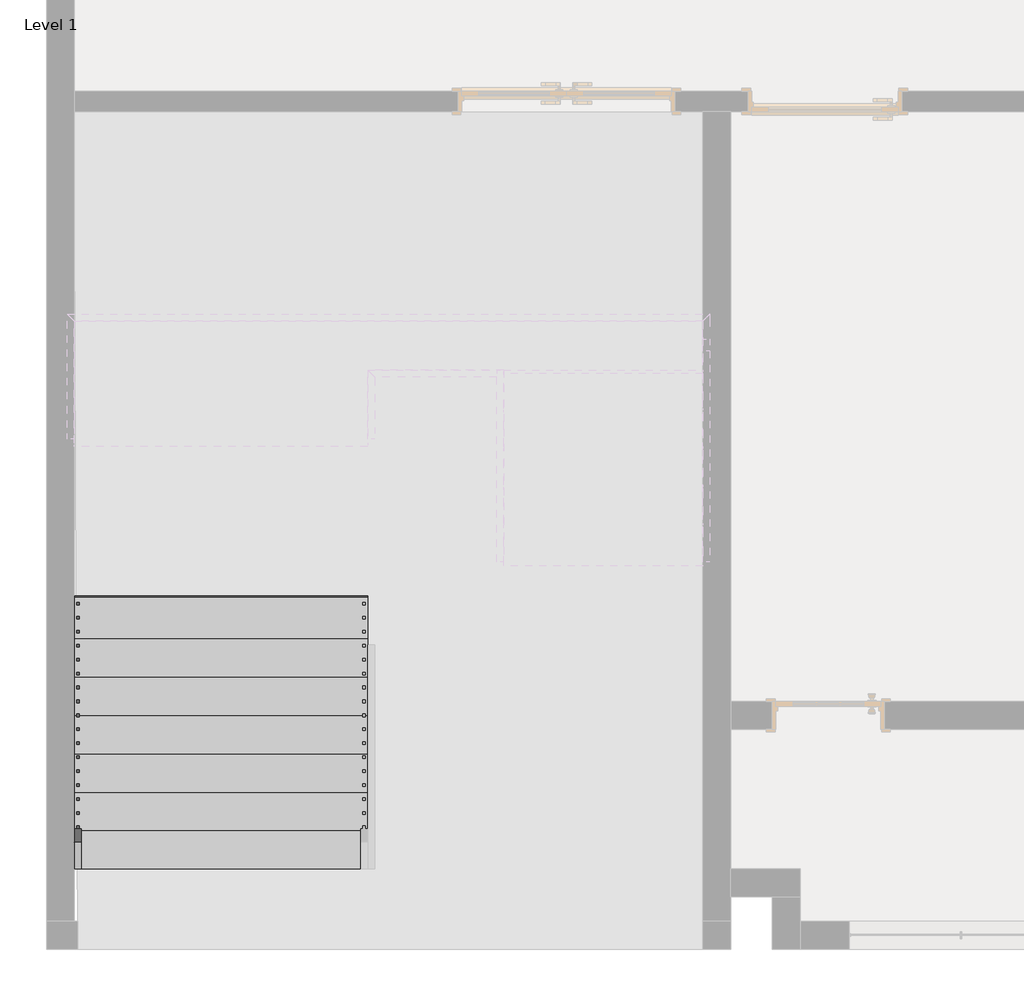
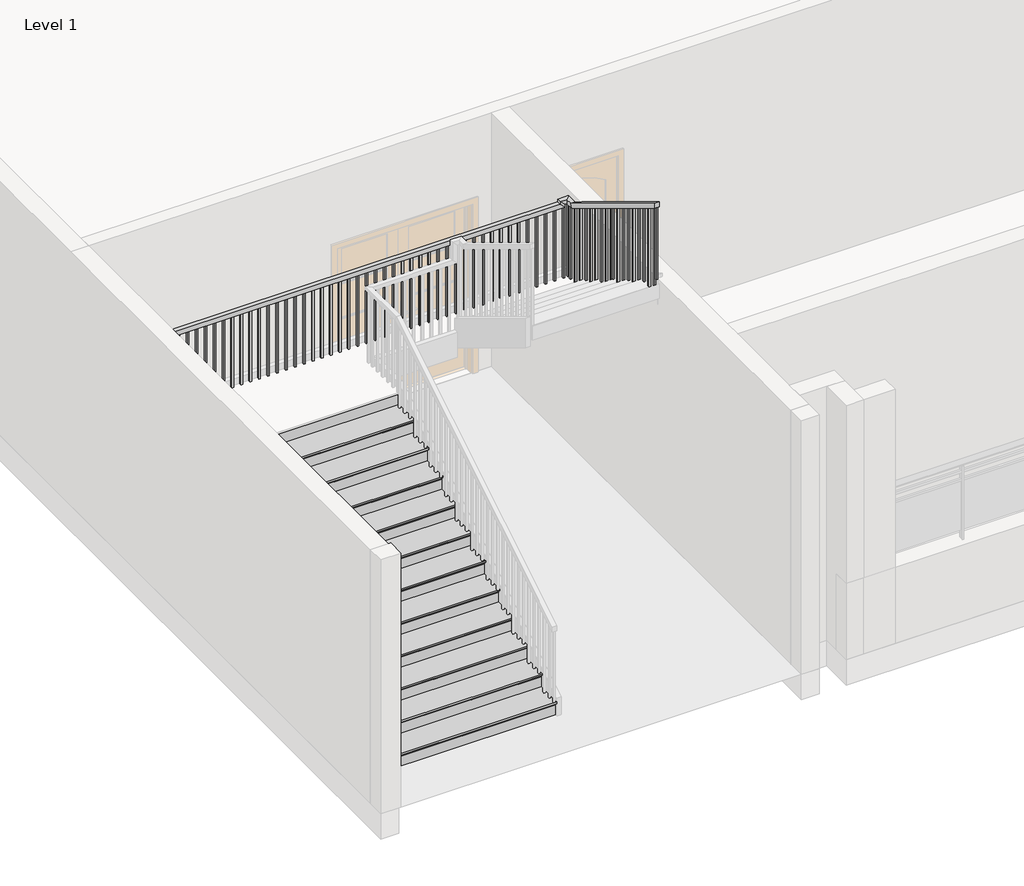
# One storey, part 3 of 4: 1 railing, 1 stair flight.
"""IFC4 building model written with IfcOpenShell, lengths in millimetres."""

from ifc_helpers import new_model, si_unit, frame, origin, place, context, project, spatial, polyline, outline, extrude, faceted_brep, transform, mapped, element, save
from components import stair_flight_3e597512

model = new_model("IFC4")

# Units and contexts
model_context = context("Model", 3, world=origin())
ifc_project = project(units=[si_unit("LENGTHUNIT", "METRE", prefix="MILLI")], contexts=[model_context])

# Site, building, storey
site = spatial("IfcSite", under=ifc_project)
building = spatial("IfcBuilding", under=site)
storey = spatial("IfcBuildingStorey", under=building, Name="Level 1", Elevation=0.0)

# Railing
placement = place(None, origin())
element("IfcRailing", 1, ObjectType="Handrail - Rectangular", at=placement, inside=storey, context=model_context, shape_type="SolidModel", body=[
    faceted_brep([(-19977.2480019, -193.7741123, 1083.7333333), (-19977.2480019, -193.7741123, 1024.3318731), (-19926.4480019, -193.7741123, 1024.3318731), (-19926.4480019, -193.7741123, 1083.7333333), (-19977.2480019, 2879.6258877, 2946.4), (-19977.2480019, 2893.8182972, 2895.6), (-19926.4480019, 2893.8182972, 2895.6), (-19926.4480019, 2879.6258877, 2946.4), (-19977.2480019, 3794.0258877, 2946.4), (-19977.2480019, 3794.0258877, 2895.6), (-19926.4480019, 3743.2258877, 2895.6), (-19926.4480019, 3743.2258877, 2946.4), (-15532.2480019, 3794.0258877, 2946.4), (-15481.4480019, 3794.0258877, 2895.6), (-15481.4480019, 3743.2258877, 2895.6), (-15532.2480019, 3743.2258877, 2946.4), (-15405.2480019, 2016.0258877, 3977.7939394), (-15456.0480019, 2016.0258877, 3977.7939394), (-15456.0480019, 2016.0258877, 3918.3924791), (-15405.2480019, 2016.0258877, 3918.3924791), (-15405.2480019, 3652.8334783, 2926.3878788), (-15405.2480019, 3667.0258877, 2977.1878788), (-15456.0480019, 3652.8334783, 2926.3878788), (-15456.0480019, 3667.0258877, 2977.1878788), (-15532.2480019, 3794.0258877, 2977.1878788), (-15481.4480019, 3794.0258877, 2926.3878788), (-15481.4480019, 3743.2258877, 2926.3878788), (-15532.2480019, 3743.2258877, 2977.1878788), (-15405.2480019, 3794.0258877, 2977.1878788), (-15405.2480019, 3794.0258877, 2926.3878788), (-15456.0480019, 3743.2258877, 2926.3878788), (-15456.0480019, 3743.2258877, 2977.1878788)], [[[0, 1, 2, 3]], [[1, 0, 4, 5]], [[2, 1, 5, 6]], [[3, 2, 6, 7]], [[0, 3, 7, 4]], [[5, 4, 8, 9]], [[6, 5, 9, 10]], [[7, 6, 10, 11]], [[4, 7, 11, 8]], [[9, 8, 12, 13]], [[10, 9, 13, 14]], [[11, 10, 14, 15]], [[8, 11, 15, 12]], [[16, 17, 18, 19]], [[20, 21, 16, 19]], [[22, 20, 19, 18]], [[23, 22, 18, 17]], [[21, 23, 17, 16]], [[13, 12, 24, 25]], [[14, 13, 25, 26]], [[15, 14, 26, 27]], [[12, 15, 27, 24]], [[25, 24, 28, 29]], [[26, 25, 29, 30]], [[27, 26, 30, 31]], [[24, 27, 31, 28]], [[29, 28, 21, 20]], [[30, 29, 20, 22]], [[31, 30, 22, 23]], [[28, 31, 23, 21]]]),
    extrude(outline(polyline([(2076.3508877, 3881.8318731), (2076.3508877, 2878.6666667), (2057.3008877, 2878.6666667), (2057.3008877, 3893.3773276), (2076.3508877, 3881.8318731)])), frame((-15440.1730019, 0.0, 0.0), z_axis=(1.0, 0.0, 0.0), x_axis=(0.0, 1.0, 0.0)), (0.0, 0.0, 1.0), 19.05),
    extrude(outline(polyline([(2177.9508877, 3820.2561155), (2177.9508877, 2878.6666667), (2158.9008877, 2878.6666667), (2158.9008877, 3831.80157), (2177.9508877, 3820.2561155)])), frame((-15440.1730019, 0.0, 0.0), z_axis=(1.0, 0.0, 0.0), x_axis=(0.0, 1.0, 0.0)), (0.0, 0.0, 1.0), 19.05),
    extrude(outline(polyline([(2279.5508877, 3758.6803579), (2279.5508877, 2878.6666667), (2260.5008877, 2878.6666667), (2260.5008877, 3770.2258125), (2279.5508877, 3758.6803579)])), frame((-15440.1730019, 0.0, 0.0), z_axis=(1.0, 0.0, 0.0), x_axis=(0.0, 1.0, 0.0)), (0.0, 0.0, 1.0), 19.05),
    extrude(outline(polyline([(2381.1508877, 3697.1046004), (2381.1508877, 2709.3333333), (2362.1008877, 2709.3333333), (2362.1008877, 3708.6500549), (2381.1508877, 3697.1046004)])), frame((-15440.1730019, 0.0, 0.0), z_axis=(1.0, 0.0, 0.0), x_axis=(0.0, 1.0, 0.0)), (0.0, 0.0, 1.0), 19.05),
    extrude(outline(polyline([(2482.7508877, 3635.5288428), (2482.7508877, 2709.3333333), (2463.7008877, 2709.3333333), (2463.7008877, 3647.0742973), (2482.7508877, 3635.5288428)])), frame((-15440.1730019, 0.0, 0.0), z_axis=(1.0, 0.0, 0.0), x_axis=(0.0, 1.0, 0.0)), (0.0, 0.0, 1.0), 19.05),
    extrude(outline(polyline([(2584.3508877, 3573.9530852), (2584.3508877, 2709.3333333), (2565.3008877, 2709.3333333), (2565.3008877, 3585.4985397), (2584.3508877, 3573.9530852)])), frame((-15440.1730019, 0.0, 0.0), z_axis=(1.0, 0.0, 0.0), x_axis=(0.0, 1.0, 0.0)), (0.0, 0.0, 1.0), 19.05),
    extrude(outline(polyline([(2685.9508877, 3512.3773276), (2685.9508877, 2540.0), (2666.9008877, 2540.0), (2666.9008877, 3523.9227822), (2685.9508877, 3512.3773276)])), frame((-15440.1730019, 0.0, 0.0), z_axis=(1.0, 0.0, 0.0), x_axis=(0.0, 1.0, 0.0)), (0.0, 0.0, 1.0), 19.05),
    extrude(outline(polyline([(2787.5508877, 3450.80157), (2787.5508877, 2540.0), (2768.5008877, 2540.0), (2768.5008877, 3462.3470246), (2787.5508877, 3450.80157)])), frame((-15440.1730019, 0.0, 0.0), z_axis=(1.0, 0.0, 0.0), x_axis=(0.0, 1.0, 0.0)), (0.0, 0.0, 1.0), 19.05),
    extrude(outline(polyline([(2914.5508877, 3373.8318731), (2914.5508877, 2370.6666667), (2895.5008877, 2370.6666667), (2895.5008877, 3385.3773276), (2914.5508877, 3373.8318731)])), frame((-15440.1730019, 0.0, 0.0), z_axis=(1.0, 0.0, 0.0), x_axis=(0.0, 1.0, 0.0)), (0.0, 0.0, 1.0), 19.05),
    extrude(outline(polyline([(3016.1508877, 3312.2561155), (3016.1508877, 2370.6666667), (2997.1008877, 2370.6666667), (2997.1008877, 3323.80157), (3016.1508877, 3312.2561155)])), frame((-15440.1730019, 0.0, 0.0), z_axis=(1.0, 0.0, 0.0), x_axis=(0.0, 1.0, 0.0)), (0.0, 0.0, 1.0), 19.05),
    extrude(outline(polyline([(3117.7508877, 3250.6803579), (3117.7508877, 2370.6666667), (3098.7008877, 2370.6666667), (3098.7008877, 3262.2258125), (3117.7508877, 3250.6803579)])), frame((-15440.1730019, 0.0, 0.0), z_axis=(1.0, 0.0, 0.0), x_axis=(0.0, 1.0, 0.0)), (0.0, 0.0, 1.0), 19.05),
    extrude(outline(polyline([(3219.3508877, 3189.1046004), (3219.3508877, 2201.3333333), (3200.3008877, 2201.3333333), (3200.3008877, 3200.6500549), (3219.3508877, 3189.1046004)])), frame((-15440.1730019, 0.0, 0.0), z_axis=(1.0, 0.0, 0.0), x_axis=(0.0, 1.0, 0.0)), (0.0, 0.0, 1.0), 19.05),
    extrude(outline(polyline([(3320.9508877, 3127.5288428), (3320.9508877, 2201.3333333), (3301.9008877, 2201.3333333), (3301.9008877, 3139.0742973), (3320.9508877, 3127.5288428)])), frame((-15440.1730019, 0.0, 0.0), z_axis=(1.0, 0.0, 0.0), x_axis=(0.0, 1.0, 0.0)), (0.0, 0.0, 1.0), 19.05),
    extrude(outline(polyline([(3422.5508877, 3065.9530852), (3422.5508877, 2201.3333333), (3403.5008877, 2201.3333333), (3403.5008877, 3077.4985397), (3422.5508877, 3065.9530852)])), frame((-15440.1730019, 0.0, 0.0), z_axis=(1.0, 0.0, 0.0), x_axis=(0.0, 1.0, 0.0)), (0.0, 0.0, 1.0), 19.05),
    extrude(outline(polyline([(3524.1508877, 3004.3773276), (3524.1508877, 2032.0), (3505.1008877, 2032.0), (3505.1008877, 3015.9227822), (3524.1508877, 3004.3773276)])), frame((-15440.1730019, 0.0, 0.0), z_axis=(1.0, 0.0, 0.0), x_axis=(0.0, 1.0, 0.0)), (0.0, 0.0, 1.0), 19.05),
    extrude(outline(polyline([(3625.7508877, 2942.80157), (3625.7508877, 2032.0), (3606.7008877, 2032.0), (3606.7008877, 2954.3470246), (3625.7508877, 2942.80157)])), frame((-15440.1730019, 0.0, 0.0), z_axis=(1.0, 0.0, 0.0), x_axis=(0.0, 1.0, 0.0)), (0.0, 0.0, 1.0), 19.05),
    extrude(outline(polyline([(-15490.9730019, 3778.1508877), (-15471.9230019, 3778.1508877), (-15471.9230019, 3759.1008877), (-15490.9730019, 3759.1008877), (-15490.9730019, 3778.1508877)])), frame((0.0, 0.0, 2032.0), z_axis=(0.0, 0.0, 1.0), x_axis=(1.0, 0.0, 0.0)), (0.0, 0.0, 1.0), 863.6),
    extrude(outline(polyline([(-15592.5730019, 3778.1508877), (-15573.5230019, 3778.1508877), (-15573.5230019, 3759.1008877), (-15592.5730019, 3759.1008877), (-15592.5730019, 3778.1508877)])), frame((0.0, 0.0, 2032.0), z_axis=(0.0, 0.0, 1.0), x_axis=(1.0, 0.0, 0.0)), (0.0, 0.0, 1.0), 863.6),
    extrude(outline(polyline([(-15694.1730019, 3778.1508877), (-15675.1230019, 3778.1508877), (-15675.1230019, 3759.1008877), (-15694.1730019, 3759.1008877), (-15694.1730019, 3778.1508877)])), frame((0.0, 0.0, 2032.0), z_axis=(0.0, 0.0, 1.0), x_axis=(1.0, 0.0, 0.0)), (0.0, 0.0, 1.0), 863.6),
    extrude(outline(polyline([(-15795.7730019, 3778.1508877), (-15776.7230019, 3778.1508877), (-15776.7230019, 3759.1008877), (-15795.7730019, 3759.1008877), (-15795.7730019, 3778.1508877)])), frame((0.0, 0.0, 2032.0), z_axis=(0.0, 0.0, 1.0), x_axis=(1.0, 0.0, 0.0)), (0.0, 0.0, 1.0), 863.6),
    extrude(outline(polyline([(-15897.3730019, 3778.1508877), (-15878.3230019, 3778.1508877), (-15878.3230019, 3759.1008877), (-15897.3730019, 3759.1008877), (-15897.3730019, 3778.1508877)])), frame((0.0, 0.0, 2032.0), z_axis=(0.0, 0.0, 1.0), x_axis=(1.0, 0.0, 0.0)), (0.0, 0.0, 1.0), 863.6),
    extrude(outline(polyline([(-15998.9730019, 3778.1508877), (-15979.9230019, 3778.1508877), (-15979.9230019, 3759.1008877), (-15998.9730019, 3759.1008877), (-15998.9730019, 3778.1508877)])), frame((0.0, 0.0, 2032.0), z_axis=(0.0, 0.0, 1.0), x_axis=(1.0, 0.0, 0.0)), (0.0, 0.0, 1.0), 863.6),
    extrude(outline(polyline([(-16100.5730019, 3778.1508877), (-16081.5230019, 3778.1508877), (-16081.5230019, 3759.1008877), (-16100.5730019, 3759.1008877), (-16100.5730019, 3778.1508877)])), frame((0.0, 0.0, 2032.0), z_axis=(0.0, 0.0, 1.0), x_axis=(1.0, 0.0, 0.0)), (0.0, 0.0, 1.0), 863.6),
    extrude(outline(polyline([(-16202.1730019, 3778.1508877), (-16183.1230019, 3778.1508877), (-16183.1230019, 3759.1008877), (-16202.1730019, 3759.1008877), (-16202.1730019, 3778.1508877)])), frame((0.0, 0.0, 2032.0), z_axis=(0.0, 0.0, 1.0), x_axis=(1.0, 0.0, 0.0)), (0.0, 0.0, 1.0), 863.6),
    extrude(outline(polyline([(-16303.7730019, 3778.1508877), (-16284.7230019, 3778.1508877), (-16284.7230019, 3759.1008877), (-16303.7730019, 3759.1008877), (-16303.7730019, 3778.1508877)])), frame((0.0, 0.0, 2032.0), z_axis=(0.0, 0.0, 1.0), x_axis=(1.0, 0.0, 0.0)), (0.0, 0.0, 1.0), 863.6),
    extrude(outline(polyline([(-16405.3730019, 3778.1508877), (-16386.3230019, 3778.1508877), (-16386.3230019, 3759.1008877), (-16405.3730019, 3759.1008877), (-16405.3730019, 3778.1508877)])), frame((0.0, 0.0, 2032.0), z_axis=(0.0, 0.0, 1.0), x_axis=(1.0, 0.0, 0.0)), (0.0, 0.0, 1.0), 863.6),
    extrude(outline(polyline([(-16506.9730019, 3778.1508877), (-16487.9230019, 3778.1508877), (-16487.9230019, 3759.1008877), (-16506.9730019, 3759.1008877), (-16506.9730019, 3778.1508877)])), frame((0.0, 0.0, 2032.0), z_axis=(0.0, 0.0, 1.0), x_axis=(1.0, 0.0, 0.0)), (0.0, 0.0, 1.0), 863.6),
    extrude(outline(polyline([(-16608.5730019, 3778.1508877), (-16589.5230019, 3778.1508877), (-16589.5230019, 3759.1008877), (-16608.5730019, 3759.1008877), (-16608.5730019, 3778.1508877)])), frame((0.0, 0.0, 2032.0), z_axis=(0.0, 0.0, 1.0), x_axis=(1.0, 0.0, 0.0)), (0.0, 0.0, 1.0), 863.6),
    extrude(outline(polyline([(-16710.1730019, 3778.1508877), (-16691.1230019, 3778.1508877), (-16691.1230019, 3759.1008877), (-16710.1730019, 3759.1008877), (-16710.1730019, 3778.1508877)])), frame((0.0, 0.0, 2032.0), z_axis=(0.0, 0.0, 1.0), x_axis=(1.0, 0.0, 0.0)), (0.0, 0.0, 1.0), 863.6),
    extrude(outline(polyline([(-16811.7730019, 3778.1508877), (-16792.7230019, 3778.1508877), (-16792.7230019, 3759.1008877), (-16811.7730019, 3759.1008877), (-16811.7730019, 3778.1508877)])), frame((0.0, 0.0, 2032.0), z_axis=(0.0, 0.0, 1.0), x_axis=(1.0, 0.0, 0.0)), (0.0, 0.0, 1.0), 863.6),
    extrude(outline(polyline([(-16913.3730019, 3778.1508877), (-16894.3230019, 3778.1508877), (-16894.3230019, 3759.1008877), (-16913.3730019, 3759.1008877), (-16913.3730019, 3778.1508877)])), frame((0.0, 0.0, 2032.0), z_axis=(0.0, 0.0, 1.0), x_axis=(1.0, 0.0, 0.0)), (0.0, 0.0, 1.0), 863.6),
    extrude(outline(polyline([(-17014.9730019, 3778.1508877), (-16995.9230019, 3778.1508877), (-16995.9230019, 3759.1008877), (-17014.9730019, 3759.1008877), (-17014.9730019, 3778.1508877)])), frame((0.0, 0.0, 2032.0), z_axis=(0.0, 0.0, 1.0), x_axis=(1.0, 0.0, 0.0)), (0.0, 0.0, 1.0), 863.6),
    extrude(outline(polyline([(-17116.5730019, 3778.1508877), (-17097.5230019, 3778.1508877), (-17097.5230019, 3759.1008877), (-17116.5730019, 3759.1008877), (-17116.5730019, 3778.1508877)])), frame((0.0, 0.0, 2032.0), z_axis=(0.0, 0.0, 1.0), x_axis=(1.0, 0.0, 0.0)), (0.0, 0.0, 1.0), 863.6),
    extrude(outline(polyline([(-17218.1730019, 3778.1508877), (-17199.1230019, 3778.1508877), (-17199.1230019, 3759.1008877), (-17218.1730019, 3759.1008877), (-17218.1730019, 3778.1508877)])), frame((0.0, 0.0, 2032.0), z_axis=(0.0, 0.0, 1.0), x_axis=(1.0, 0.0, 0.0)), (0.0, 0.0, 1.0), 863.6),
    extrude(outline(polyline([(-17319.7730019, 3778.1508877), (-17300.7230019, 3778.1508877), (-17300.7230019, 3759.1008877), (-17319.7730019, 3759.1008877), (-17319.7730019, 3778.1508877)])), frame((0.0, 0.0, 2032.0), z_axis=(0.0, 0.0, 1.0), x_axis=(1.0, 0.0, 0.0)), (0.0, 0.0, 1.0), 863.6),
    extrude(outline(polyline([(-17421.3730019, 3778.1508877), (-17402.3230019, 3778.1508877), (-17402.3230019, 3759.1008877), (-17421.3730019, 3759.1008877), (-17421.3730019, 3778.1508877)])), frame((0.0, 0.0, 2032.0), z_axis=(0.0, 0.0, 1.0), x_axis=(1.0, 0.0, 0.0)), (0.0, 0.0, 1.0), 863.6),
    extrude(outline(polyline([(-17522.9730019, 3778.1508877), (-17503.9230019, 3778.1508877), (-17503.9230019, 3759.1008877), (-17522.9730019, 3759.1008877), (-17522.9730019, 3778.1508877)])), frame((0.0, 0.0, 2032.0), z_axis=(0.0, 0.0, 1.0), x_axis=(1.0, 0.0, 0.0)), (0.0, 0.0, 1.0), 863.6),
    extrude(outline(polyline([(-17624.5730019, 3778.1508877), (-17605.5230019, 3778.1508877), (-17605.5230019, 3759.1008877), (-17624.5730019, 3759.1008877), (-17624.5730019, 3778.1508877)])), frame((0.0, 0.0, 2032.0), z_axis=(0.0, 0.0, 1.0), x_axis=(1.0, 0.0, 0.0)), (0.0, 0.0, 1.0), 863.6),
    extrude(outline(polyline([(-17726.1730019, 3778.1508877), (-17707.1230019, 3778.1508877), (-17707.1230019, 3759.1008877), (-17726.1730019, 3759.1008877), (-17726.1730019, 3778.1508877)])), frame((0.0, 0.0, 2032.0), z_axis=(0.0, 0.0, 1.0), x_axis=(1.0, 0.0, 0.0)), (0.0, 0.0, 1.0), 863.6),
    extrude(outline(polyline([(-17827.7730019, 3778.1508877), (-17808.7230019, 3778.1508877), (-17808.7230019, 3759.1008877), (-17827.7730019, 3759.1008877), (-17827.7730019, 3778.1508877)])), frame((0.0, 0.0, 2032.0), z_axis=(0.0, 0.0, 1.0), x_axis=(1.0, 0.0, 0.0)), (0.0, 0.0, 1.0), 863.6),
    extrude(outline(polyline([(-17929.3730019, 3778.1508877), (-17910.3230019, 3778.1508877), (-17910.3230019, 3759.1008877), (-17929.3730019, 3759.1008877), (-17929.3730019, 3778.1508877)])), frame((0.0, 0.0, 2032.0), z_axis=(0.0, 0.0, 1.0), x_axis=(1.0, 0.0, 0.0)), (0.0, 0.0, 1.0), 863.6),
    extrude(outline(polyline([(-18030.9730019, 3778.1508877), (-18011.9230019, 3778.1508877), (-18011.9230019, 3759.1008877), (-18030.9730019, 3759.1008877), (-18030.9730019, 3778.1508877)])), frame((0.0, 0.0, 2032.0), z_axis=(0.0, 0.0, 1.0), x_axis=(1.0, 0.0, 0.0)), (0.0, 0.0, 1.0), 863.6),
    extrude(outline(polyline([(-18132.5730019, 3778.1508877), (-18113.5230019, 3778.1508877), (-18113.5230019, 3759.1008877), (-18132.5730019, 3759.1008877), (-18132.5730019, 3778.1508877)])), frame((0.0, 0.0, 2032.0), z_axis=(0.0, 0.0, 1.0), x_axis=(1.0, 0.0, 0.0)), (0.0, 0.0, 1.0), 863.6),
    extrude(outline(polyline([(-18234.1730019, 3778.1508877), (-18215.1230019, 3778.1508877), (-18215.1230019, 3759.1008877), (-18234.1730019, 3759.1008877), (-18234.1730019, 3778.1508877)])), frame((0.0, 0.0, 2032.0), z_axis=(0.0, 0.0, 1.0), x_axis=(1.0, 0.0, 0.0)), (0.0, 0.0, 1.0), 863.6),
    extrude(outline(polyline([(-18335.7730019, 3778.1508877), (-18316.7230019, 3778.1508877), (-18316.7230019, 3759.1008877), (-18335.7730019, 3759.1008877), (-18335.7730019, 3778.1508877)])), frame((0.0, 0.0, 2032.0), z_axis=(0.0, 0.0, 1.0), x_axis=(1.0, 0.0, 0.0)), (0.0, 0.0, 1.0), 863.6),
    extrude(outline(polyline([(-18437.3730019, 3778.1508877), (-18418.3230019, 3778.1508877), (-18418.3230019, 3759.1008877), (-18437.3730019, 3759.1008877), (-18437.3730019, 3778.1508877)])), frame((0.0, 0.0, 2032.0), z_axis=(0.0, 0.0, 1.0), x_axis=(1.0, 0.0, 0.0)), (0.0, 0.0, 1.0), 863.6),
    extrude(outline(polyline([(-18538.9730019, 3778.1508877), (-18519.9230019, 3778.1508877), (-18519.9230019, 3759.1008877), (-18538.9730019, 3759.1008877), (-18538.9730019, 3778.1508877)])), frame((0.0, 0.0, 2032.0), z_axis=(0.0, 0.0, 1.0), x_axis=(1.0, 0.0, 0.0)), (0.0, 0.0, 1.0), 863.6),
    extrude(outline(polyline([(-18640.5730019, 3778.1508877), (-18621.5230019, 3778.1508877), (-18621.5230019, 3759.1008877), (-18640.5730019, 3759.1008877), (-18640.5730019, 3778.1508877)])), frame((0.0, 0.0, 2032.0), z_axis=(0.0, 0.0, 1.0), x_axis=(1.0, 0.0, 0.0)), (0.0, 0.0, 1.0), 863.6),
    extrude(outline(polyline([(-18742.1730019, 3778.1508877), (-18723.1230019, 3778.1508877), (-18723.1230019, 3759.1008877), (-18742.1730019, 3759.1008877), (-18742.1730019, 3778.1508877)])), frame((0.0, 0.0, 2032.0), z_axis=(0.0, 0.0, 1.0), x_axis=(1.0, 0.0, 0.0)), (0.0, 0.0, 1.0), 863.6),
    extrude(outline(polyline([(-18843.7730019, 3778.1508877), (-18824.7230019, 3778.1508877), (-18824.7230019, 3759.1008877), (-18843.7730019, 3759.1008877), (-18843.7730019, 3778.1508877)])), frame((0.0, 0.0, 2032.0), z_axis=(0.0, 0.0, 1.0), x_axis=(1.0, 0.0, 0.0)), (0.0, 0.0, 1.0), 863.6),
    extrude(outline(polyline([(-18945.3730019, 3778.1508877), (-18926.3230019, 3778.1508877), (-18926.3230019, 3759.1008877), (-18945.3730019, 3759.1008877), (-18945.3730019, 3778.1508877)])), frame((0.0, 0.0, 2032.0), z_axis=(0.0, 0.0, 1.0), x_axis=(1.0, 0.0, 0.0)), (0.0, 0.0, 1.0), 863.6),
    extrude(outline(polyline([(-19046.9730019, 3778.1508877), (-19027.9230019, 3778.1508877), (-19027.9230019, 3759.1008877), (-19046.9730019, 3759.1008877), (-19046.9730019, 3778.1508877)])), frame((0.0, 0.0, 2032.0), z_axis=(0.0, 0.0, 1.0), x_axis=(1.0, 0.0, 0.0)), (0.0, 0.0, 1.0), 863.6),
    extrude(outline(polyline([(-19148.5730019, 3778.1508877), (-19129.5230019, 3778.1508877), (-19129.5230019, 3759.1008877), (-19148.5730019, 3759.1008877), (-19148.5730019, 3778.1508877)])), frame((0.0, 0.0, 2032.0), z_axis=(0.0, 0.0, 1.0), x_axis=(1.0, 0.0, 0.0)), (0.0, 0.0, 1.0), 863.6),
    extrude(outline(polyline([(-19250.1730019, 3778.1508877), (-19231.1230019, 3778.1508877), (-19231.1230019, 3759.1008877), (-19250.1730019, 3759.1008877), (-19250.1730019, 3778.1508877)])), frame((0.0, 0.0, 2032.0), z_axis=(0.0, 0.0, 1.0), x_axis=(1.0, 0.0, 0.0)), (0.0, 0.0, 1.0), 863.6),
    extrude(outline(polyline([(-19351.7730019, 3778.1508877), (-19332.7230019, 3778.1508877), (-19332.7230019, 3759.1008877), (-19351.7730019, 3759.1008877), (-19351.7730019, 3778.1508877)])), frame((0.0, 0.0, 2032.0), z_axis=(0.0, 0.0, 1.0), x_axis=(1.0, 0.0, 0.0)), (0.0, 0.0, 1.0), 863.6),
    extrude(outline(polyline([(-19453.3730019, 3778.1508877), (-19434.3230019, 3778.1508877), (-19434.3230019, 3759.1008877), (-19453.3730019, 3759.1008877), (-19453.3730019, 3778.1508877)])), frame((0.0, 0.0, 2032.0), z_axis=(0.0, 0.0, 1.0), x_axis=(1.0, 0.0, 0.0)), (0.0, 0.0, 1.0), 863.6),
    extrude(outline(polyline([(-19554.9730019, 3778.1508877), (-19535.9230019, 3778.1508877), (-19535.9230019, 3759.1008877), (-19554.9730019, 3759.1008877), (-19554.9730019, 3778.1508877)])), frame((0.0, 0.0, 2032.0), z_axis=(0.0, 0.0, 1.0), x_axis=(1.0, 0.0, 0.0)), (0.0, 0.0, 1.0), 863.6),
    extrude(outline(polyline([(-19656.5730019, 3778.1508877), (-19637.5230019, 3778.1508877), (-19637.5230019, 3759.1008877), (-19656.5730019, 3759.1008877), (-19656.5730019, 3778.1508877)])), frame((0.0, 0.0, 2032.0), z_axis=(0.0, 0.0, 1.0), x_axis=(1.0, 0.0, 0.0)), (0.0, 0.0, 1.0), 863.6),
    extrude(outline(polyline([(-19758.1730019, 3778.1508877), (-19739.1230019, 3778.1508877), (-19739.1230019, 3759.1008877), (-19758.1730019, 3759.1008877), (-19758.1730019, 3778.1508877)])), frame((0.0, 0.0, 2032.0), z_axis=(0.0, 0.0, 1.0), x_axis=(1.0, 0.0, 0.0)), (0.0, 0.0, 1.0), 863.6),
    extrude(outline(polyline([(-19859.7730019, 3778.1508877), (-19840.7230019, 3778.1508877), (-19840.7230019, 3759.1008877), (-19859.7730019, 3759.1008877), (-19859.7730019, 3778.1508877)])), frame((0.0, 0.0, 2032.0), z_axis=(0.0, 0.0, 1.0), x_axis=(1.0, 0.0, 0.0)), (0.0, 0.0, 1.0), 863.6),
    extrude(outline(polyline([(-19961.3730019, 3682.9008877), (-19961.3730019, 3701.9508877), (-19942.3230019, 3701.9508877), (-19942.3230019, 3682.9008877), (-19961.3730019, 3682.9008877)])), frame((0.0, 0.0, 2032.0), z_axis=(0.0, 0.0, 1.0), x_axis=(1.0, 0.0, 0.0)), (0.0, 0.0, 1.0), 863.6),
    extrude(outline(polyline([(-19961.3730019, 3581.3008877), (-19961.3730019, 3600.3508877), (-19942.3230019, 3600.3508877), (-19942.3230019, 3581.3008877), (-19961.3730019, 3581.3008877)])), frame((0.0, 0.0, 2032.0), z_axis=(0.0, 0.0, 1.0), x_axis=(1.0, 0.0, 0.0)), (0.0, 0.0, 1.0), 863.6),
    extrude(outline(polyline([(-19961.3730019, 3479.7008877), (-19961.3730019, 3498.7508877), (-19942.3230019, 3498.7508877), (-19942.3230019, 3479.7008877), (-19961.3730019, 3479.7008877)])), frame((0.0, 0.0, 2032.0), z_axis=(0.0, 0.0, 1.0), x_axis=(1.0, 0.0, 0.0)), (0.0, 0.0, 1.0), 863.6),
    extrude(outline(polyline([(-19961.3730019, 3378.1008877), (-19961.3730019, 3397.1508877), (-19942.3230019, 3397.1508877), (-19942.3230019, 3378.1008877), (-19961.3730019, 3378.1008877)])), frame((0.0, 0.0, 2032.0), z_axis=(0.0, 0.0, 1.0), x_axis=(1.0, 0.0, 0.0)), (0.0, 0.0, 1.0), 863.6),
    extrude(outline(polyline([(-19961.3730019, 3276.5008877), (-19961.3730019, 3295.5508877), (-19942.3230019, 3295.5508877), (-19942.3230019, 3276.5008877), (-19961.3730019, 3276.5008877)])), frame((0.0, 0.0, 2032.0), z_axis=(0.0, 0.0, 1.0), x_axis=(1.0, 0.0, 0.0)), (0.0, 0.0, 1.0), 863.6),
    extrude(outline(polyline([(-19961.3730019, 3174.9008877), (-19961.3730019, 3193.9508877), (-19942.3230019, 3193.9508877), (-19942.3230019, 3174.9008877), (-19961.3730019, 3174.9008877)])), frame((0.0, 0.0, 2032.0), z_axis=(0.0, 0.0, 1.0), x_axis=(1.0, 0.0, 0.0)), (0.0, 0.0, 1.0), 863.6),
    extrude(outline(polyline([(-19961.3730019, 3073.3008877), (-19961.3730019, 3092.3508877), (-19942.3230019, 3092.3508877), (-19942.3230019, 3073.3008877), (-19961.3730019, 3073.3008877)])), frame((0.0, 0.0, 2032.0), z_axis=(0.0, 0.0, 1.0), x_axis=(1.0, 0.0, 0.0)), (0.0, 0.0, 1.0), 863.6),
    extrude(outline(polyline([(-19961.3730019, 2971.7008877), (-19961.3730019, 2990.7508877), (-19942.3230019, 2990.7508877), (-19942.3230019, 2971.7008877), (-19961.3730019, 2971.7008877)])), frame((0.0, 0.0, 2032.0), z_axis=(0.0, 0.0, 1.0), x_axis=(1.0, 0.0, 0.0)), (0.0, 0.0, 1.0), 863.6),
    extrude(outline(polyline([(2863.7508877, 2877.3773276), (2863.7508877, 1862.6666667), (2844.7008877, 1862.6666667), (2844.7008877, 2865.8318731), (2863.7508877, 2877.3773276)])), frame((-19961.3730019, 0.0, 0.0), z_axis=(1.0, 0.0, 0.0), x_axis=(0.0, 1.0, 0.0)), (0.0, 0.0, 1.0), 19.05),
    extrude(outline(polyline([(2762.1508877, 2815.80157), (2762.1508877, 1862.6666667), (2743.1008877, 1862.6666667), (2743.1008877, 2804.2561155), (2762.1508877, 2815.80157)])), frame((-19961.3730019, 0.0, 0.0), z_axis=(1.0, 0.0, 0.0), x_axis=(0.0, 1.0, 0.0)), (0.0, 0.0, 1.0), 19.05),
    extrude(outline(polyline([(2660.5508877, 2754.2258125), (2660.5508877, 1862.6666667), (2641.5008877, 1862.6666667), (2641.5008877, 2742.6803579), (2660.5508877, 2754.2258125)])), frame((-19961.3730019, 0.0, 0.0), z_axis=(1.0, 0.0, 0.0), x_axis=(0.0, 1.0, 0.0)), (0.0, 0.0, 1.0), 19.05),
    extrude(outline(polyline([(2558.9508877, 2692.6500549), (2558.9508877, 1693.3333333), (2539.9008877, 1693.3333333), (2539.9008877, 2681.1046004), (2558.9508877, 2692.6500549)])), frame((-19961.3730019, 0.0, 0.0), z_axis=(1.0, 0.0, 0.0), x_axis=(0.0, 1.0, 0.0)), (0.0, 0.0, 1.0), 19.05),
    extrude(outline(polyline([(2457.3508877, 2631.0742973), (2457.3508877, 1693.3333333), (2438.3008877, 1693.3333333), (2438.3008877, 2619.5288428), (2457.3508877, 2631.0742973)])), frame((-19961.3730019, 0.0, 0.0), z_axis=(1.0, 0.0, 0.0), x_axis=(0.0, 1.0, 0.0)), (0.0, 0.0, 1.0), 19.05),
    extrude(outline(polyline([(2355.7508877, 2569.4985397), (2355.7508877, 1693.3333333), (2336.7008877, 1693.3333333), (2336.7008877, 2557.9530852), (2355.7508877, 2569.4985397)])), frame((-19961.3730019, 0.0, 0.0), z_axis=(1.0, 0.0, 0.0), x_axis=(0.0, 1.0, 0.0)), (0.0, 0.0, 1.0), 19.05),
    extrude(outline(polyline([(2254.1508877, 2507.9227822), (2254.1508877, 1524.0), (2235.1008877, 1524.0), (2235.1008877, 2496.3773276), (2254.1508877, 2507.9227822)])), frame((-19961.3730019, 0.0, 0.0), z_axis=(1.0, 0.0, 0.0), x_axis=(0.0, 1.0, 0.0)), (0.0, 0.0, 1.0), 19.05),
    extrude(outline(polyline([(2152.5508877, 2446.3470246), (2152.5508877, 1524.0), (2133.5008877, 1524.0), (2133.5008877, 2434.80157), (2152.5508877, 2446.3470246)])), frame((-19961.3730019, 0.0, 0.0), z_axis=(1.0, 0.0, 0.0), x_axis=(0.0, 1.0, 0.0)), (0.0, 0.0, 1.0), 19.05),
    extrude(outline(polyline([(2050.9508877, 2384.771267), (2050.9508877, 1524.0), (2031.9008877, 1524.0), (2031.9008877, 2373.2258125), (2050.9508877, 2384.771267)])), frame((-19961.3730019, 0.0, 0.0), z_axis=(1.0, 0.0, 0.0), x_axis=(0.0, 1.0, 0.0)), (0.0, 0.0, 1.0), 19.05),
    extrude(outline(polyline([(1949.3508877, 2323.1955094), (1949.3508877, 1354.6666667), (1930.3008877, 1354.6666667), (1930.3008877, 2311.6500549), (1949.3508877, 2323.1955094)])), frame((-19961.3730019, 0.0, 0.0), z_axis=(1.0, 0.0, 0.0), x_axis=(0.0, 1.0, 0.0)), (0.0, 0.0, 1.0), 19.05),
    extrude(outline(polyline([(1847.7508877, 2261.6197519), (1847.7508877, 1354.6666667), (1828.7008877, 1354.6666667), (1828.7008877, 2250.0742973), (1847.7508877, 2261.6197519)])), frame((-19961.3730019, 0.0, 0.0), z_axis=(1.0, 0.0, 0.0), x_axis=(0.0, 1.0, 0.0)), (0.0, 0.0, 1.0), 19.05),
    extrude(outline(polyline([(1746.1508877, 2200.0439943), (1746.1508877, 1185.3333333), (1727.1008877, 1185.3333333), (1727.1008877, 2188.4985397), (1746.1508877, 2200.0439943)])), frame((-19961.3730019, 0.0, 0.0), z_axis=(1.0, 0.0, 0.0), x_axis=(0.0, 1.0, 0.0)), (0.0, 0.0, 1.0), 19.05),
    extrude(outline(polyline([(1644.5508877, 2138.4682367), (1644.5508877, 1185.3333333), (1625.5008877, 1185.3333333), (1625.5008877, 2126.9227822), (1644.5508877, 2138.4682367)])), frame((-19961.3730019, 0.0, 0.0), z_axis=(1.0, 0.0, 0.0), x_axis=(0.0, 1.0, 0.0)), (0.0, 0.0, 1.0), 19.05),
    extrude(outline(polyline([(1542.9508877, 2076.8924791), (1542.9508877, 1185.3333333), (1523.9008877, 1185.3333333), (1523.9008877, 2065.3470246), (1542.9508877, 2076.8924791)])), frame((-19961.3730019, 0.0, 0.0), z_axis=(1.0, 0.0, 0.0), x_axis=(0.0, 1.0, 0.0)), (0.0, 0.0, 1.0), 19.05),
    extrude(outline(polyline([(1441.3508877, 2015.3167216), (1441.3508877, 1016.0), (1422.3008877, 1016.0), (1422.3008877, 2003.771267), (1441.3508877, 2015.3167216)])), frame((-19961.3730019, 0.0, 0.0), z_axis=(1.0, 0.0, 0.0), x_axis=(0.0, 1.0, 0.0)), (0.0, 0.0, 1.0), 19.05),
    extrude(outline(polyline([(1339.7508877, 1953.740964), (1339.7508877, 1016.0), (1320.7008877, 1016.0), (1320.7008877, 1942.1955094), (1339.7508877, 1953.740964)])), frame((-19961.3730019, 0.0, 0.0), z_axis=(1.0, 0.0, 0.0), x_axis=(0.0, 1.0, 0.0)), (0.0, 0.0, 1.0), 19.05),
    extrude(outline(polyline([(1238.1508877, 1892.1652064), (1238.1508877, 1016.0), (1219.1008877, 1016.0), (1219.1008877, 1880.6197519), (1238.1508877, 1892.1652064)])), frame((-19961.3730019, 0.0, 0.0), z_axis=(1.0, 0.0, 0.0), x_axis=(0.0, 1.0, 0.0)), (0.0, 0.0, 1.0), 19.05),
    extrude(outline(polyline([(1136.5508877, 1830.5894488), (1136.5508877, 846.6666667), (1117.5008877, 846.6666667), (1117.5008877, 1819.0439943), (1136.5508877, 1830.5894488)])), frame((-19961.3730019, 0.0, 0.0), z_axis=(1.0, 0.0, 0.0), x_axis=(0.0, 1.0, 0.0)), (0.0, 0.0, 1.0), 19.05),
    extrude(outline(polyline([(1034.9508877, 1769.0136913), (1034.9508877, 846.6666667), (1015.9008877, 846.6666667), (1015.9008877, 1757.4682367), (1034.9508877, 1769.0136913)])), frame((-19961.3730019, 0.0, 0.0), z_axis=(1.0, 0.0, 0.0), x_axis=(0.0, 1.0, 0.0)), (0.0, 0.0, 1.0), 19.05),
    extrude(outline(polyline([(933.3508877, 1707.4379337), (933.3508877, 846.6666667), (914.3008877, 846.6666667), (914.3008877, 1695.8924791), (933.3508877, 1707.4379337)])), frame((-19961.3730019, 0.0, 0.0), z_axis=(1.0, 0.0, 0.0), x_axis=(0.0, 1.0, 0.0)), (0.0, 0.0, 1.0), 19.05),
    extrude(outline(polyline([(831.7508877, 1645.8621761), (831.7508877, 677.3333333), (812.7008877, 677.3333333), (812.7008877, 1634.3167216), (831.7508877, 1645.8621761)])), frame((-19961.3730019, 0.0, 0.0), z_axis=(1.0, 0.0, 0.0), x_axis=(0.0, 1.0, 0.0)), (0.0, 0.0, 1.0), 19.05),
    extrude(outline(polyline([(730.1508877, 1584.2864185), (730.1508877, 677.3333333), (711.1008877, 677.3333333), (711.1008877, 1572.740964), (730.1508877, 1584.2864185)])), frame((-19961.3730019, 0.0, 0.0), z_axis=(1.0, 0.0, 0.0), x_axis=(0.0, 1.0, 0.0)), (0.0, 0.0, 1.0), 19.05),
    extrude(outline(polyline([(628.5508877, 1522.710661), (628.5508877, 508.0), (609.5008877, 508.0), (609.5008877, 1511.1652064), (628.5508877, 1522.710661)])), frame((-19961.3730019, 0.0, 0.0), z_axis=(1.0, 0.0, 0.0), x_axis=(0.0, 1.0, 0.0)), (0.0, 0.0, 1.0), 19.05),
    extrude(outline(polyline([(526.9508877, 1461.1349034), (526.9508877, 508.0), (507.9008877, 508.0), (507.9008877, 1449.5894488), (526.9508877, 1461.1349034)])), frame((-19961.3730019, 0.0, 0.0), z_axis=(1.0, 0.0, 0.0), x_axis=(0.0, 1.0, 0.0)), (0.0, 0.0, 1.0), 19.05),
    extrude(outline(polyline([(425.3508877, 1399.5591458), (425.3508877, 508.0), (406.3008877, 508.0), (406.3008877, 1388.0136913), (425.3508877, 1399.5591458)])), frame((-19961.3730019, 0.0, 0.0), z_axis=(1.0, 0.0, 0.0), x_axis=(0.0, 1.0, 0.0)), (0.0, 0.0, 1.0), 19.05),
    extrude(outline(polyline([(323.7508877, 1337.9833882), (323.7508877, 338.6666667), (304.7008877, 338.6666667), (304.7008877, 1326.4379337), (323.7508877, 1337.9833882)])), frame((-19961.3730019, 0.0, 0.0), z_axis=(1.0, 0.0, 0.0), x_axis=(0.0, 1.0, 0.0)), (0.0, 0.0, 1.0), 19.05),
    extrude(outline(polyline([(222.1508877, 1276.4076307), (222.1508877, 338.6666667), (203.1008877, 338.6666667), (203.1008877, 1264.8621761), (222.1508877, 1276.4076307)])), frame((-19961.3730019, 0.0, 0.0), z_axis=(1.0, 0.0, 0.0), x_axis=(0.0, 1.0, 0.0)), (0.0, 0.0, 1.0), 19.05),
    extrude(outline(polyline([(120.5508877, 1214.8318731), (120.5508877, 338.6666667), (101.5008877, 338.6666667), (101.5008877, 1203.2864185), (120.5508877, 1214.8318731)])), frame((-19961.3730019, 0.0, 0.0), z_axis=(1.0, 0.0, 0.0), x_axis=(0.0, 1.0, 0.0)), (0.0, 0.0, 1.0), 19.05),
    extrude(outline(polyline([(18.9508877, 1153.2561155), (18.9508877, 169.3333333), (-0.0991123, 169.3333333), (-0.0991123, 1141.710661), (18.9508877, 1153.2561155)])), frame((-19961.3730019, 0.0, 0.0), z_axis=(1.0, 0.0, 0.0), x_axis=(0.0, 1.0, 0.0)), (0.0, 0.0, 1.0), 19.05),
    extrude(outline(polyline([(-82.6491123, 1091.6803579), (-82.6491123, 169.3333333), (-101.6991123, 169.3333333), (-101.6991123, 1080.1349034), (-82.6491123, 1091.6803579)])), frame((-19961.3730019, 0.0, 0.0), z_axis=(1.0, 0.0, 0.0), x_axis=(0.0, 1.0, 0.0)), (0.0, 0.0, 1.0), 19.05),
    extrude(outline(polyline([(2889.1508877, 3389.2258125), (2889.1508877, 2540.0), (2870.1008877, 2540.0), (2870.1008877, 3400.771267), (2889.1508877, 3389.2258125)])), frame((-15440.1730019, 0.0, 0.0), z_axis=(1.0, 0.0, 0.0), x_axis=(0.0, 1.0, 0.0)), (0.0, 0.0, 1.0), 19.05),
    extrude(outline(polyline([(-15421.1230019, 3727.3508877), (-15421.1230019, 3708.3008877), (-15440.1730019, 3708.3008877), (-15440.1730019, 3727.3508877), (-15421.1230019, 3727.3508877)])), frame((0.0, 0.0, 2032.0), z_axis=(0.0, 0.0, 1.0), x_axis=(1.0, 0.0, 0.0)), (0.0, 0.0, 1.0), 894.3878788),
    extrude(outline(polyline([(-15440.1730019, 3778.1508877), (-15421.1230019, 3778.1508877), (-15421.1230019, 3759.1008877), (-15440.1730019, 3759.1008877), (-15440.1730019, 3778.1508877)])), frame((0.0, 0.0, 2032.0), z_axis=(0.0, 0.0, 1.0), x_axis=(1.0, 0.0, 0.0)), (0.0, 0.0, 1.0), 894.3878788),
    extrude(outline(polyline([(-19961.3730019, 3759.1008877), (-19961.3730019, 3778.1508877), (-19942.3230019, 3778.1508877), (-19942.3230019, 3759.1008877), (-19961.3730019, 3759.1008877)])), frame((0.0, 0.0, 2032.0), z_axis=(0.0, 0.0, 1.0), x_axis=(1.0, 0.0, 0.0)), (0.0, 0.0, 1.0), 863.6),
    extrude(outline(polyline([(-19961.3730019, 2870.1008877), (-19961.3730019, 2889.1508877), (-19942.3230019, 2889.1508877), (-19942.3230019, 2870.1008877), (-19961.3730019, 2870.1008877)])), frame((0.0, 0.0, 2032.0), z_axis=(0.0, 0.0, 1.0), x_axis=(1.0, 0.0, 0.0)), (0.0, 0.0, 1.0), 863.6),
    extrude(outline(polyline([(2035.0758877, 3906.8470246), (2035.0758877, 3057.6212121), (2016.0258877, 3057.6212121), (2016.0258877, 3918.3924791), (2035.0758877, 3906.8470246)])), frame((-15440.1730019, 0.0, 0.0), z_axis=(1.0, 0.0, 0.0), x_axis=(0.0, 1.0, 0.0)), (0.0, 0.0, 1.0), 19.05),
    extrude(outline(polyline([(-174.7241123, 1035.8773276), (-174.7241123, 169.3333333), (-193.7741123, 169.3333333), (-193.7741123, 1024.3318731), (-174.7241123, 1035.8773276)])), frame((-19961.3730019, 0.0, 0.0), z_axis=(1.0, 0.0, 0.0), x_axis=(0.0, 1.0, 0.0)), (0.0, 0.0, 1.0), 19.05),
])

# Stair flight
stair_flight_shape = stair_flight_3e597512(model_context)
element("IfcStairFlight", 2, ObjectType="2\" Tread 1\" Nosing 1/4\" Riser", at=placement, inside=storey, context=model_context, shape_type="MappedRepresentation", body=[
    mapped(stair_flight_shape, transform((0.0, 0.0, 0.0), x_axis=(1.0, 0.0, 0.0), y_axis=(0.0, 1.0, 0.0), z_axis=(0.0, 0.0, 1.0))),
])

save(model, "model.ifc")

# Revit data of these elements
# Type "Handrail - Rectangular"
#   Assembly Code = "C2010400"
#   built-in parameter 1008612 = 0.0416667 (stored number, unit not read)
#   built-in parameter 1008611 = 0.0416667 (stored number, unit not read)
#   built-in parameter 1008609 = 0.333333 (stored number, unit not read)
#   built-in parameter 1008604 = 0.166667 (stored number, unit not read)
#   built-in parameter 1008603 = 0.166667 (stored number, unit not read)
#   Railing Height = 3' - 0"
#   built-in parameter 1008630 = 2
#   built-in parameter 1008610 = 2
#   built-in parameter 1008618 = Baluster - Square : 3/4"
# Element 1 (IfcRailing, "Handrail - Rectangular")
#   Phase Created = New Construction
# Element 2 (IfcStairFlight, "2\" Tread 1\" Nosing 1/4\" Riser")
#   Phase Created = New Construction
